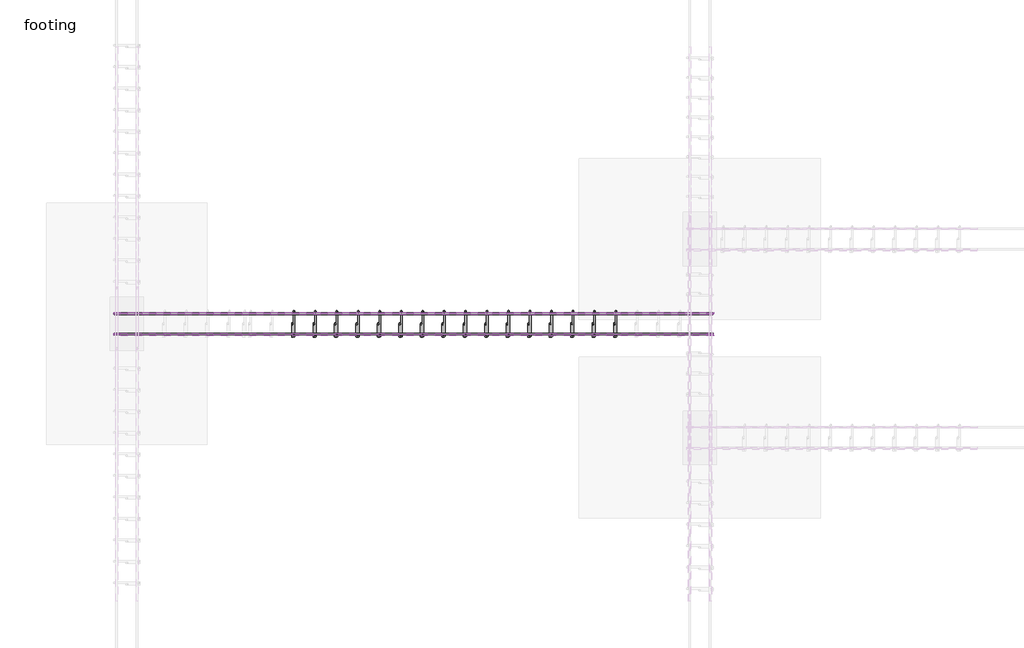
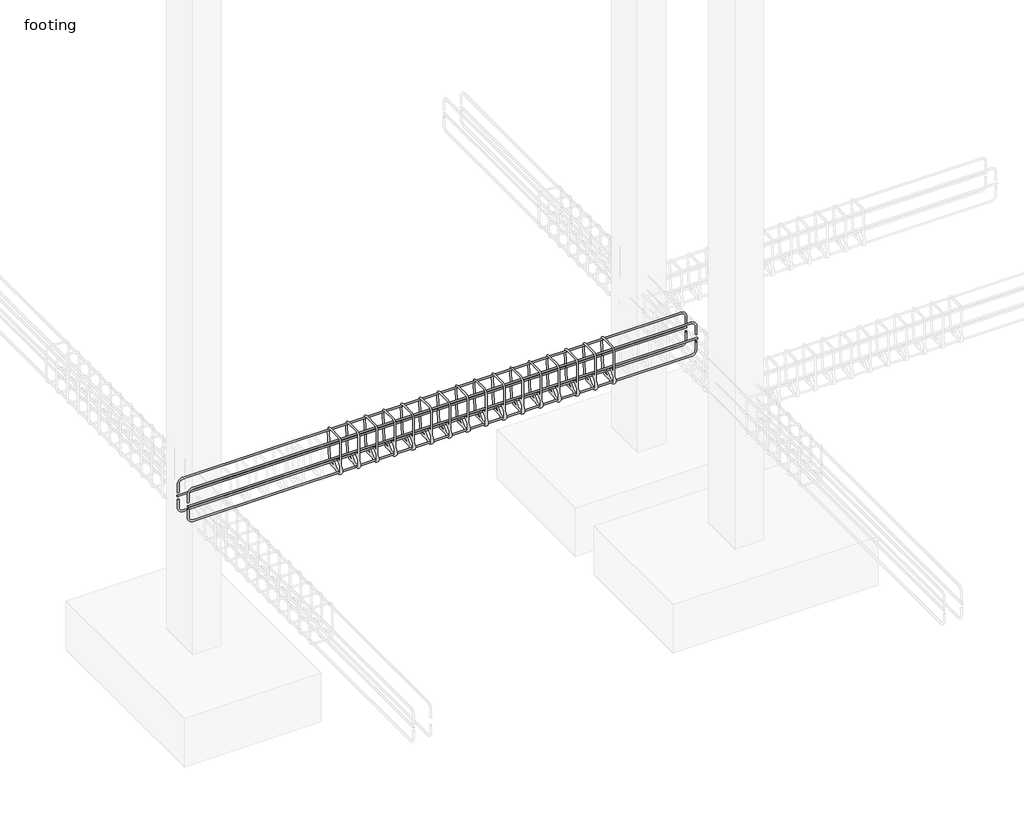
# One storey, part 8 of 21: 22 reinforcing bars.
"""IFC4 building model written with IfcOpenShell, lengths in millimetres."""

from ifc_helpers import new_model, si_unit, point, frame, origin, place, context, project, spatial, polyline, circle_curve, trimmed, segment, composite_curve, element, save
from ifc_brep_helpers import swept_disk

model = new_model("IFC4")

# Units and contexts
model_context = context("Model", 3, world=origin())
ifc_project = project(units=[si_unit("LENGTHUNIT", "METRE", prefix="MILLI")], contexts=[model_context])

# Site, building, storey
site = spatial("IfcSite", under=ifc_project)
building = spatial("IfcBuilding", under=site)
storey = spatial("IfcBuildingStorey", under=building, Name="footing", Elevation=-1524.0)

# Reinforcing bars
placement = place(None, origin())
element("IfcReinforcingBar", 1, at=placement, inside=storey, context=model_context, shape_type="SolidModel", body=[
    swept_disk(composite_curve([segment(polyline([(-10956.0883428, 7572.2887132, -310.8825168), (-10956.0883428, 7517.4237147, -365.7475153)]), True, "CONTINUOUS"), segment(trimmed(circle_curve(frame((-10956.0883428, 7494.9730744, -343.296875), z_axis=(-1.0, 0.0, 0.0), x_axis=(0.0, 22.450640300000487, -22.450640299999975)), 31.75), [point((-10956.0883428, 7517.4237147, -365.7475153))], [point((-10956.0883428, 7463.2230744, -343.296875))], True, "CARTESIAN"), True, "CONTINUOUS"), segment(polyline([(-10956.0883428, 7463.2230744, -343.296875), (-10956.0883428, 7463.2230744, -63.103125)]), True, "CONTINUOUS"), segment(trimmed(circle_curve(frame((-10956.0883428, 7494.9730744, -63.103125), z_axis=(-1.0, 0.0, 0.0), x_axis=(0.0, -31.75, 0.0)), 31.75), [point((-10956.0883428, 7463.2230744, -63.103125))], [point((-10956.0883428, 7494.9730744, -31.353125))], True, "CARTESIAN"), True, "CONTINUOUS"), segment(polyline([(-10956.0883428, 7494.9730744, -31.353125), (-10956.0883428, 7622.7668244, -31.353125)]), True, "CONTINUOUS"), segment(trimmed(circle_curve(frame((-10954.9159328, 7622.7668244, -63.0814712), z_axis=(-0.9993179916193466, 0.0, -0.03692629992126919), x_axis=(-1.1724099999992177, 0.0, 31.728346200000004)), 31.75), [point((-10956.0883428, 7622.7668244, -31.353125))], [point((-10954.9159328, 7654.5168244, -63.0814712))], True, "CARTESIAN"), True, "CONTINUOUS"), segment(polyline([(-10954.9159328, 7654.5168244, -63.0814712), (-10944.5607528, 7654.5168244, -343.3185288)]), True, "CONTINUOUS"), segment(trimmed(circle_curve(frame((-10944.5607528, 7622.7668244, -343.3185288), z_axis=(-0.9993179916193466, 0.0, -0.03692629992126919), x_axis=(0.0, 31.75, 0.0)), 31.75), [point((-10944.5607528, 7654.5168244, -343.3185288))], [point((-10943.3883428, 7622.7668244, -375.046875))], True, "CARTESIAN"), True, "CONTINUOUS"), segment(polyline([(-10943.3883428, 7622.7668244, -375.046875), (-10943.3883428, 7494.9730744, -375.046875)]), True, "CONTINUOUS"), segment(trimmed(circle_curve(frame((-10943.3883428, 7494.9730744, -343.296875), z_axis=(-1.0, 0.0, 0.0), x_axis=(0.0, 0.0, -31.75)), 31.75), [point((-10943.3883428, 7494.9730744, -375.046875))], [point((-10943.3883428, 7472.5224341, -320.8462347))], True, "CARTESIAN"), True, "CONTINUOUS"), segment(polyline([(-10943.3883428, 7472.5224341, -320.8462347), (-10943.3883428, 7527.3874326, -265.9812362)]), True, "CONTINUOUS")], self_intersect=False), 6.35),
])
element("IfcReinforcingBar", 2, at=placement, inside=storey, context=model_context, shape_type="SolidModel", body=[
    swept_disk(composite_curve([segment(polyline([(-10793.3883428, 7572.2887132, -310.8825168), (-10793.3883428, 7517.4237147, -365.7475153)]), True, "CONTINUOUS"), segment(trimmed(circle_curve(frame((-10793.3883428, 7494.9730744, -343.296875), z_axis=(-1.0, 0.0, 0.0), x_axis=(0.0, 22.450640300000487, -22.450640299999975)), 31.75), [point((-10793.3883428, 7517.4237147, -365.7475153))], [point((-10793.3883428, 7463.2230744, -343.296875))], True, "CARTESIAN"), True, "CONTINUOUS"), segment(polyline([(-10793.3883428, 7463.2230744, -343.296875), (-10793.3883428, 7463.2230744, -63.103125)]), True, "CONTINUOUS"), segment(trimmed(circle_curve(frame((-10793.3883428, 7494.9730744, -63.103125), z_axis=(-1.0, 0.0, 0.0), x_axis=(0.0, -31.75, 0.0)), 31.75), [point((-10793.3883428, 7463.2230744, -63.103125))], [point((-10793.3883428, 7494.9730744, -31.353125))], True, "CARTESIAN"), True, "CONTINUOUS"), segment(polyline([(-10793.3883428, 7494.9730744, -31.353125), (-10793.3883428, 7622.7668244, -31.353125)]), True, "CONTINUOUS"), segment(trimmed(circle_curve(frame((-10792.2159328, 7622.7668244, -63.0814712), z_axis=(-0.9993179916193466, 0.0, -0.03692629992126919), x_axis=(-1.1724100000010367, 0.0, 31.728346200000004)), 31.75), [point((-10793.3883428, 7622.7668244, -31.353125))], [point((-10792.2159328, 7654.5168244, -63.0814712))], True, "CARTESIAN"), True, "CONTINUOUS"), segment(polyline([(-10792.2159328, 7654.5168244, -63.0814712), (-10781.8607528, 7654.5168244, -343.3185288)]), True, "CONTINUOUS"), segment(trimmed(circle_curve(frame((-10781.8607528, 7622.7668244, -343.3185288), z_axis=(-0.9993179916193466, 0.0, -0.03692629992126919), x_axis=(0.0, 31.75, 0.0)), 31.75), [point((-10781.8607528, 7654.5168244, -343.3185288))], [point((-10780.6883428, 7622.7668244, -375.046875))], True, "CARTESIAN"), True, "CONTINUOUS"), segment(polyline([(-10780.6883428, 7622.7668244, -375.046875), (-10780.6883428, 7494.9730744, -375.046875)]), True, "CONTINUOUS"), segment(trimmed(circle_curve(frame((-10780.6883428, 7494.9730744, -343.296875), z_axis=(-1.0, 0.0, 0.0), x_axis=(0.0, 0.0, -31.75)), 31.75), [point((-10780.6883428, 7494.9730744, -375.046875))], [point((-10780.6883428, 7472.5224341, -320.8462347))], True, "CARTESIAN"), True, "CONTINUOUS"), segment(polyline([(-10780.6883428, 7472.5224341, -320.8462347), (-10780.6883428, 7527.3874326, -265.9812362)]), True, "CONTINUOUS")], self_intersect=False), 6.35),
])
element("IfcReinforcingBar", 3, at=placement, inside=storey, context=model_context, shape_type="SolidModel", body=[
    swept_disk(composite_curve([segment(polyline([(-10630.6883428, 7572.2887132, -310.8825168), (-10630.6883428, 7517.4237147, -365.7475153)]), True, "CONTINUOUS"), segment(trimmed(circle_curve(frame((-10630.6883428, 7494.9730744, -343.296875), z_axis=(-1.0, 0.0, 0.0), x_axis=(0.0, 22.450640300000487, -22.450640299999975)), 31.75), [point((-10630.6883428, 7517.4237147, -365.7475153))], [point((-10630.6883428, 7463.2230744, -343.296875))], True, "CARTESIAN"), True, "CONTINUOUS"), segment(polyline([(-10630.6883428, 7463.2230744, -343.296875), (-10630.6883428, 7463.2230744, -63.103125)]), True, "CONTINUOUS"), segment(trimmed(circle_curve(frame((-10630.6883428, 7494.9730744, -63.103125), z_axis=(-1.0, 0.0, 0.0), x_axis=(0.0, -31.75, 0.0)), 31.75), [point((-10630.6883428, 7463.2230744, -63.103125))], [point((-10630.6883428, 7494.9730744, -31.353125))], True, "CARTESIAN"), True, "CONTINUOUS"), segment(polyline([(-10630.6883428, 7494.9730744, -31.353125), (-10630.6883428, 7622.7668244, -31.353125)]), True, "CONTINUOUS"), segment(trimmed(circle_curve(frame((-10629.5159328, 7622.7668244, -63.0814712), z_axis=(-0.9993179916193466, 0.0, -0.03692629992126919), x_axis=(-1.1724099999992177, 0.0, 31.728346200000004)), 31.75), [point((-10630.6883428, 7622.7668244, -31.353125))], [point((-10629.5159328, 7654.5168244, -63.0814712))], True, "CARTESIAN"), True, "CONTINUOUS"), segment(polyline([(-10629.5159328, 7654.5168244, -63.0814712), (-10619.1607528, 7654.5168244, -343.3185288)]), True, "CONTINUOUS"), segment(trimmed(circle_curve(frame((-10619.1607528, 7622.7668244, -343.3185288), z_axis=(-0.9993179916193466, 0.0, -0.03692629992126919), x_axis=(0.0, 31.75, 0.0)), 31.75), [point((-10619.1607528, 7654.5168244, -343.3185288))], [point((-10617.9883428, 7622.7668244, -375.046875))], True, "CARTESIAN"), True, "CONTINUOUS"), segment(polyline([(-10617.9883428, 7622.7668244, -375.046875), (-10617.9883428, 7494.9730744, -375.046875)]), True, "CONTINUOUS"), segment(trimmed(circle_curve(frame((-10617.9883428, 7494.9730744, -343.296875), z_axis=(-1.0, 0.0, 0.0), x_axis=(0.0, 0.0, -31.75)), 31.75), [point((-10617.9883428, 7494.9730744, -375.046875))], [point((-10617.9883428, 7472.5224341, -320.8462347))], True, "CARTESIAN"), True, "CONTINUOUS"), segment(polyline([(-10617.9883428, 7472.5224341, -320.8462347), (-10617.9883428, 7527.3874326, -265.9812362)]), True, "CONTINUOUS")], self_intersect=False), 6.35),
])
element("IfcReinforcingBar", 4, at=placement, inside=storey, context=model_context, shape_type="SolidModel", body=[
    swept_disk(composite_curve([segment(polyline([(-10467.9883428, 7572.2887132, -310.8825168), (-10467.9883428, 7517.4237147, -365.7475153)]), True, "CONTINUOUS"), segment(trimmed(circle_curve(frame((-10467.9883428, 7494.9730744, -343.296875), z_axis=(-1.0, 0.0, 0.0), x_axis=(0.0, 22.450640300000487, -22.450640299999975)), 31.75), [point((-10467.9883428, 7517.4237147, -365.7475153))], [point((-10467.9883428, 7463.2230744, -343.296875))], True, "CARTESIAN"), True, "CONTINUOUS"), segment(polyline([(-10467.9883428, 7463.2230744, -343.296875), (-10467.9883428, 7463.2230744, -63.103125)]), True, "CONTINUOUS"), segment(trimmed(circle_curve(frame((-10467.9883428, 7494.9730744, -63.103125), z_axis=(-1.0, 0.0, 0.0), x_axis=(0.0, -31.75, 0.0)), 31.75), [point((-10467.9883428, 7463.2230744, -63.103125))], [point((-10467.9883428, 7494.9730744, -31.353125))], True, "CARTESIAN"), True, "CONTINUOUS"), segment(polyline([(-10467.9883428, 7494.9730744, -31.353125), (-10467.9883428, 7622.7668244, -31.353125)]), True, "CONTINUOUS"), segment(trimmed(circle_curve(frame((-10466.8159328, 7622.7668244, -63.0814712), z_axis=(-0.9993179916193466, 0.0, -0.03692629992126919), x_axis=(-1.1724099999992177, 0.0, 31.728346200000004)), 31.75), [point((-10467.9883428, 7622.7668244, -31.353125))], [point((-10466.8159328, 7654.5168244, -63.0814712))], True, "CARTESIAN"), True, "CONTINUOUS"), segment(polyline([(-10466.8159328, 7654.5168244, -63.0814712), (-10456.4607528, 7654.5168244, -343.3185288)]), True, "CONTINUOUS"), segment(trimmed(circle_curve(frame((-10456.4607528, 7622.7668244, -343.3185288), z_axis=(-0.9993179916193466, 0.0, -0.03692629992126919), x_axis=(0.0, 31.75, 0.0)), 31.75), [point((-10456.4607528, 7654.5168244, -343.3185288))], [point((-10455.2883428, 7622.7668244, -375.046875))], True, "CARTESIAN"), True, "CONTINUOUS"), segment(polyline([(-10455.2883428, 7622.7668244, -375.046875), (-10455.2883428, 7494.9730744, -375.046875)]), True, "CONTINUOUS"), segment(trimmed(circle_curve(frame((-10455.2883428, 7494.9730744, -343.296875), z_axis=(-1.0, 0.0, 0.0), x_axis=(0.0, 0.0, -31.75)), 31.75), [point((-10455.2883428, 7494.9730744, -375.046875))], [point((-10455.2883428, 7472.5224341, -320.8462347))], True, "CARTESIAN"), True, "CONTINUOUS"), segment(polyline([(-10455.2883428, 7472.5224341, -320.8462347), (-10455.2883428, 7527.3874326, -265.9812362)]), True, "CONTINUOUS")], self_intersect=False), 6.35),
])
element("IfcReinforcingBar", 5, at=placement, inside=storey, context=model_context, shape_type="SolidModel", body=[
    swept_disk(composite_curve([segment(polyline([(-10305.2883428, 7572.2887132, -310.8825168), (-10305.2883428, 7517.4237147, -365.7475153)]), True, "CONTINUOUS"), segment(trimmed(circle_curve(frame((-10305.2883428, 7494.9730744, -343.296875), z_axis=(-1.0, 0.0, 0.0), x_axis=(0.0, 22.450640300000487, -22.450640299999975)), 31.75), [point((-10305.2883428, 7517.4237147, -365.7475153))], [point((-10305.2883428, 7463.2230744, -343.296875))], True, "CARTESIAN"), True, "CONTINUOUS"), segment(polyline([(-10305.2883428, 7463.2230744, -343.296875), (-10305.2883428, 7463.2230744, -63.103125)]), True, "CONTINUOUS"), segment(trimmed(circle_curve(frame((-10305.2883428, 7494.9730744, -63.103125), z_axis=(-1.0, 0.0, 0.0), x_axis=(0.0, -31.75, 0.0)), 31.75), [point((-10305.2883428, 7463.2230744, -63.103125))], [point((-10305.2883428, 7494.9730744, -31.353125))], True, "CARTESIAN"), True, "CONTINUOUS"), segment(polyline([(-10305.2883428, 7494.9730744, -31.353125), (-10305.2883428, 7622.7668244, -31.353125)]), True, "CONTINUOUS"), segment(trimmed(circle_curve(frame((-10304.1159328, 7622.7668244, -63.0814712), z_axis=(-0.9993179916193466, 0.0, -0.03692629992126919), x_axis=(-1.1724100000010367, 0.0, 31.728346200000004)), 31.75), [point((-10305.2883428, 7622.7668244, -31.353125))], [point((-10304.1159328, 7654.5168244, -63.0814712))], True, "CARTESIAN"), True, "CONTINUOUS"), segment(polyline([(-10304.1159328, 7654.5168244, -63.0814712), (-10293.7607528, 7654.5168244, -343.3185288)]), True, "CONTINUOUS"), segment(trimmed(circle_curve(frame((-10293.7607528, 7622.7668244, -343.3185288), z_axis=(-0.9993179916193466, 0.0, -0.03692629992126919), x_axis=(0.0, 31.75, 0.0)), 31.75), [point((-10293.7607528, 7654.5168244, -343.3185288))], [point((-10292.5883428, 7622.7668244, -375.046875))], True, "CARTESIAN"), True, "CONTINUOUS"), segment(polyline([(-10292.5883428, 7622.7668244, -375.046875), (-10292.5883428, 7494.9730744, -375.046875)]), True, "CONTINUOUS"), segment(trimmed(circle_curve(frame((-10292.5883428, 7494.9730744, -343.296875), z_axis=(-1.0, 0.0, 0.0), x_axis=(0.0, 0.0, -31.75)), 31.75), [point((-10292.5883428, 7494.9730744, -375.046875))], [point((-10292.5883428, 7472.5224341, -320.8462347))], True, "CARTESIAN"), True, "CONTINUOUS"), segment(polyline([(-10292.5883428, 7472.5224341, -320.8462347), (-10292.5883428, 7527.3874326, -265.9812362)]), True, "CONTINUOUS")], self_intersect=False), 6.35),
])
element("IfcReinforcingBar", 6, at=placement, inside=storey, context=model_context, shape_type="SolidModel", body=[
    swept_disk(composite_curve([segment(polyline([(-10142.5883428, 7572.2887132, -310.8825168), (-10142.5883428, 7517.4237147, -365.7475153)]), True, "CONTINUOUS"), segment(trimmed(circle_curve(frame((-10142.5883428, 7494.9730744, -343.296875), z_axis=(-1.0, 0.0, 0.0), x_axis=(0.0, 22.450640300000487, -22.450640299999975)), 31.75), [point((-10142.5883428, 7517.4237147, -365.7475153))], [point((-10142.5883428, 7463.2230744, -343.296875))], True, "CARTESIAN"), True, "CONTINUOUS"), segment(polyline([(-10142.5883428, 7463.2230744, -343.296875), (-10142.5883428, 7463.2230744, -63.103125)]), True, "CONTINUOUS"), segment(trimmed(circle_curve(frame((-10142.5883428, 7494.9730744, -63.103125), z_axis=(-1.0, 0.0, 0.0), x_axis=(0.0, -31.75, 0.0)), 31.75), [point((-10142.5883428, 7463.2230744, -63.103125))], [point((-10142.5883428, 7494.9730744, -31.353125))], True, "CARTESIAN"), True, "CONTINUOUS"), segment(polyline([(-10142.5883428, 7494.9730744, -31.353125), (-10142.5883428, 7622.7668244, -31.353125)]), True, "CONTINUOUS"), segment(trimmed(circle_curve(frame((-10141.4159328, 7622.7668244, -63.0814712), z_axis=(-0.9993179916193466, 0.0, -0.03692629992126919), x_axis=(-1.1724099999992177, 0.0, 31.728346200000004)), 31.75), [point((-10142.5883428, 7622.7668244, -31.353125))], [point((-10141.4159328, 7654.5168244, -63.0814712))], True, "CARTESIAN"), True, "CONTINUOUS"), segment(polyline([(-10141.4159328, 7654.5168244, -63.0814712), (-10131.0607528, 7654.5168244, -343.3185288)]), True, "CONTINUOUS"), segment(trimmed(circle_curve(frame((-10131.0607528, 7622.7668244, -343.3185288), z_axis=(-0.9993179916193466, 0.0, -0.03692629992126919), x_axis=(0.0, 31.75, 0.0)), 31.75), [point((-10131.0607528, 7654.5168244, -343.3185288))], [point((-10129.8883428, 7622.7668244, -375.046875))], True, "CARTESIAN"), True, "CONTINUOUS"), segment(polyline([(-10129.8883428, 7622.7668244, -375.046875), (-10129.8883428, 7494.9730744, -375.046875)]), True, "CONTINUOUS"), segment(trimmed(circle_curve(frame((-10129.8883428, 7494.9730744, -343.296875), z_axis=(-1.0, 0.0, 0.0), x_axis=(0.0, 0.0, -31.75)), 31.75), [point((-10129.8883428, 7494.9730744, -375.046875))], [point((-10129.8883428, 7472.5224341, -320.8462347))], True, "CARTESIAN"), True, "CONTINUOUS"), segment(polyline([(-10129.8883428, 7472.5224341, -320.8462347), (-10129.8883428, 7527.3874326, -265.9812362)]), True, "CONTINUOUS")], self_intersect=False), 6.35),
])
element("IfcReinforcingBar", 7, at=placement, inside=storey, context=model_context, shape_type="SolidModel", body=[
    swept_disk(composite_curve([segment(polyline([(-9979.8883428, 7572.2887132, -310.8825168), (-9979.8883428, 7517.4237147, -365.7475153)]), True, "CONTINUOUS"), segment(trimmed(circle_curve(frame((-9979.8883428, 7494.9730744, -343.296875), z_axis=(-1.0, 0.0, 0.0), x_axis=(0.0, 22.450640300000487, -22.450640299999975)), 31.75), [point((-9979.8883428, 7517.4237147, -365.7475153))], [point((-9979.8883428, 7463.2230744, -343.296875))], True, "CARTESIAN"), True, "CONTINUOUS"), segment(polyline([(-9979.8883428, 7463.2230744, -343.296875), (-9979.8883428, 7463.2230744, -63.103125)]), True, "CONTINUOUS"), segment(trimmed(circle_curve(frame((-9979.8883428, 7494.9730744, -63.103125), z_axis=(-1.0, 0.0, 0.0), x_axis=(0.0, -31.75, 0.0)), 31.75), [point((-9979.8883428, 7463.2230744, -63.103125))], [point((-9979.8883428, 7494.9730744, -31.353125))], True, "CARTESIAN"), True, "CONTINUOUS"), segment(polyline([(-9979.8883428, 7494.9730744, -31.353125), (-9979.8883428, 7622.7668244, -31.353125)]), True, "CONTINUOUS"), segment(trimmed(circle_curve(frame((-9978.7159328, 7622.7668244, -63.0814712), z_axis=(-0.9993179916193466, 0.0, -0.03692629992126919), x_axis=(-1.1724100000010367, 0.0, 31.728346200000004)), 31.75), [point((-9979.8883428, 7622.7668244, -31.353125))], [point((-9978.7159328, 7654.5168244, -63.0814712))], True, "CARTESIAN"), True, "CONTINUOUS"), segment(polyline([(-9978.7159328, 7654.5168244, -63.0814712), (-9968.3607528, 7654.5168244, -343.3185288)]), True, "CONTINUOUS"), segment(trimmed(circle_curve(frame((-9968.3607528, 7622.7668244, -343.3185288), z_axis=(-0.9993179916193466, 0.0, -0.03692629992126919), x_axis=(0.0, 31.75, 0.0)), 31.75), [point((-9968.3607528, 7654.5168244, -343.3185288))], [point((-9967.1883428, 7622.7668244, -375.046875))], True, "CARTESIAN"), True, "CONTINUOUS"), segment(polyline([(-9967.1883428, 7622.7668244, -375.046875), (-9967.1883428, 7494.9730744, -375.046875)]), True, "CONTINUOUS"), segment(trimmed(circle_curve(frame((-9967.1883428, 7494.9730744, -343.296875), z_axis=(-1.0, 0.0, 0.0), x_axis=(0.0, 0.0, -31.75)), 31.75), [point((-9967.1883428, 7494.9730744, -375.046875))], [point((-9967.1883428, 7472.5224341, -320.8462347))], True, "CARTESIAN"), True, "CONTINUOUS"), segment(polyline([(-9967.1883428, 7472.5224341, -320.8462347), (-9967.1883428, 7527.3874326, -265.9812362)]), True, "CONTINUOUS")], self_intersect=False), 6.35),
])
element("IfcReinforcingBar", 8, at=placement, inside=storey, context=model_context, shape_type="SolidModel", body=[
    swept_disk(composite_curve([segment(polyline([(-9817.1883428, 7572.2887132, -310.8825168), (-9817.1883428, 7517.4237147, -365.7475153)]), True, "CONTINUOUS"), segment(trimmed(circle_curve(frame((-9817.1883428, 7494.9730744, -343.296875), z_axis=(-1.0, 0.0, 0.0), x_axis=(0.0, 22.450640300000487, -22.450640299999975)), 31.75), [point((-9817.1883428, 7517.4237147, -365.7475153))], [point((-9817.1883428, 7463.2230744, -343.296875))], True, "CARTESIAN"), True, "CONTINUOUS"), segment(polyline([(-9817.1883428, 7463.2230744, -343.296875), (-9817.1883428, 7463.2230744, -63.103125)]), True, "CONTINUOUS"), segment(trimmed(circle_curve(frame((-9817.1883428, 7494.9730744, -63.103125), z_axis=(-1.0, 0.0, 0.0), x_axis=(0.0, -31.75, 0.0)), 31.75), [point((-9817.1883428, 7463.2230744, -63.103125))], [point((-9817.1883428, 7494.9730744, -31.353125))], True, "CARTESIAN"), True, "CONTINUOUS"), segment(polyline([(-9817.1883428, 7494.9730744, -31.353125), (-9817.1883428, 7622.7668244, -31.353125)]), True, "CONTINUOUS"), segment(trimmed(circle_curve(frame((-9816.0159328, 7622.7668244, -63.0814712), z_axis=(-0.9993179916193466, 0.0, -0.03692629992126919), x_axis=(-1.1724099999992177, 0.0, 31.728346200000004)), 31.75), [point((-9817.1883428, 7622.7668244, -31.353125))], [point((-9816.0159328, 7654.5168244, -63.0814712))], True, "CARTESIAN"), True, "CONTINUOUS"), segment(polyline([(-9816.0159328, 7654.5168244, -63.0814712), (-9805.6607528, 7654.5168244, -343.3185288)]), True, "CONTINUOUS"), segment(trimmed(circle_curve(frame((-9805.6607528, 7622.7668244, -343.3185288), z_axis=(-0.9993179916193466, 0.0, -0.03692629992126919), x_axis=(0.0, 31.75, 0.0)), 31.75), [point((-9805.6607528, 7654.5168244, -343.3185288))], [point((-9804.4883428, 7622.7668244, -375.046875))], True, "CARTESIAN"), True, "CONTINUOUS"), segment(polyline([(-9804.4883428, 7622.7668244, -375.046875), (-9804.4883428, 7494.9730744, -375.046875)]), True, "CONTINUOUS"), segment(trimmed(circle_curve(frame((-9804.4883428, 7494.9730744, -343.296875), z_axis=(-1.0, 0.0, 0.0), x_axis=(0.0, 0.0, -31.75)), 31.75), [point((-9804.4883428, 7494.9730744, -375.046875))], [point((-9804.4883428, 7472.5224341, -320.8462347))], True, "CARTESIAN"), True, "CONTINUOUS"), segment(polyline([(-9804.4883428, 7472.5224341, -320.8462347), (-9804.4883428, 7527.3874326, -265.9812362)]), True, "CONTINUOUS")], self_intersect=False), 6.35),
])
element("IfcReinforcingBar", 9, at=placement, inside=storey, context=model_context, shape_type="SolidModel", body=[
    swept_disk(composite_curve([segment(polyline([(-9654.4883428, 7572.2887132, -310.8825168), (-9654.4883428, 7517.4237147, -365.7475153)]), True, "CONTINUOUS"), segment(trimmed(circle_curve(frame((-9654.4883428, 7494.9730744, -343.296875), z_axis=(-1.0, 0.0, 0.0), x_axis=(0.0, 22.450640300000487, -22.450640299999975)), 31.75), [point((-9654.4883428, 7517.4237147, -365.7475153))], [point((-9654.4883428, 7463.2230744, -343.296875))], True, "CARTESIAN"), True, "CONTINUOUS"), segment(polyline([(-9654.4883428, 7463.2230744, -343.296875), (-9654.4883428, 7463.2230744, -63.103125)]), True, "CONTINUOUS"), segment(trimmed(circle_curve(frame((-9654.4883428, 7494.9730744, -63.103125), z_axis=(-1.0, 0.0, 0.0), x_axis=(0.0, -31.75, 0.0)), 31.75), [point((-9654.4883428, 7463.2230744, -63.103125))], [point((-9654.4883428, 7494.9730744, -31.353125))], True, "CARTESIAN"), True, "CONTINUOUS"), segment(polyline([(-9654.4883428, 7494.9730744, -31.353125), (-9654.4883428, 7622.7668244, -31.353125)]), True, "CONTINUOUS"), segment(trimmed(circle_curve(frame((-9653.3159328, 7622.7668244, -63.0814712), z_axis=(-0.9993179916193466, 0.0, -0.03692629992126919), x_axis=(-1.1724099999992177, 0.0, 31.728346200000004)), 31.75), [point((-9654.4883428, 7622.7668244, -31.353125))], [point((-9653.3159328, 7654.5168244, -63.0814712))], True, "CARTESIAN"), True, "CONTINUOUS"), segment(polyline([(-9653.3159328, 7654.5168244, -63.0814712), (-9642.9607528, 7654.5168244, -343.3185288)]), True, "CONTINUOUS"), segment(trimmed(circle_curve(frame((-9642.9607528, 7622.7668244, -343.3185288), z_axis=(-0.9993179916193466, 0.0, -0.03692629992126919), x_axis=(0.0, 31.75, 0.0)), 31.75), [point((-9642.9607528, 7654.5168244, -343.3185288))], [point((-9641.7883428, 7622.7668244, -375.046875))], True, "CARTESIAN"), True, "CONTINUOUS"), segment(polyline([(-9641.7883428, 7622.7668244, -375.046875), (-9641.7883428, 7494.9730744, -375.046875)]), True, "CONTINUOUS"), segment(trimmed(circle_curve(frame((-9641.7883428, 7494.9730744, -343.296875), z_axis=(-1.0, 0.0, 0.0), x_axis=(0.0, 0.0, -31.75)), 31.75), [point((-9641.7883428, 7494.9730744, -375.046875))], [point((-9641.7883428, 7472.5224341, -320.8462347))], True, "CARTESIAN"), True, "CONTINUOUS"), segment(polyline([(-9641.7883428, 7472.5224341, -320.8462347), (-9641.7883428, 7527.3874326, -265.9812362)]), True, "CONTINUOUS")], self_intersect=False), 6.35),
])
element("IfcReinforcingBar", 10, at=placement, inside=storey, context=model_context, shape_type="SolidModel", body=[
    swept_disk(composite_curve([segment(polyline([(-9491.7883428, 7572.2887132, -310.8825168), (-9491.7883428, 7517.4237147, -365.7475153)]), True, "CONTINUOUS"), segment(trimmed(circle_curve(frame((-9491.7883428, 7494.9730744, -343.296875), z_axis=(-1.0, 0.0, 0.0), x_axis=(0.0, 22.450640300000487, -22.450640299999975)), 31.75), [point((-9491.7883428, 7517.4237147, -365.7475153))], [point((-9491.7883428, 7463.2230744, -343.296875))], True, "CARTESIAN"), True, "CONTINUOUS"), segment(polyline([(-9491.7883428, 7463.2230744, -343.296875), (-9491.7883428, 7463.2230744, -63.103125)]), True, "CONTINUOUS"), segment(trimmed(circle_curve(frame((-9491.7883428, 7494.9730744, -63.103125), z_axis=(-1.0, 0.0, 0.0), x_axis=(0.0, -31.75, 0.0)), 31.75), [point((-9491.7883428, 7463.2230744, -63.103125))], [point((-9491.7883428, 7494.9730744, -31.353125))], True, "CARTESIAN"), True, "CONTINUOUS"), segment(polyline([(-9491.7883428, 7494.9730744, -31.353125), (-9491.7883428, 7622.7668244, -31.353125)]), True, "CONTINUOUS"), segment(trimmed(circle_curve(frame((-9490.6159328, 7622.7668244, -63.0814712), z_axis=(-0.9993179916193466, 0.0, -0.03692629992126919), x_axis=(-1.1724100000010367, 0.0, 31.728346200000004)), 31.75), [point((-9491.7883428, 7622.7668244, -31.353125))], [point((-9490.6159328, 7654.5168244, -63.0814712))], True, "CARTESIAN"), True, "CONTINUOUS"), segment(polyline([(-9490.6159328, 7654.5168244, -63.0814712), (-9480.2607528, 7654.5168244, -343.3185288)]), True, "CONTINUOUS"), segment(trimmed(circle_curve(frame((-9480.2607528, 7622.7668244, -343.3185288), z_axis=(-0.9993179916193466, 0.0, -0.03692629992126919), x_axis=(0.0, 31.75, 0.0)), 31.75), [point((-9480.2607528, 7654.5168244, -343.3185288))], [point((-9479.0883428, 7622.7668244, -375.046875))], True, "CARTESIAN"), True, "CONTINUOUS"), segment(polyline([(-9479.0883428, 7622.7668244, -375.046875), (-9479.0883428, 7494.9730744, -375.046875)]), True, "CONTINUOUS"), segment(trimmed(circle_curve(frame((-9479.0883428, 7494.9730744, -343.296875), z_axis=(-1.0, 0.0, 0.0), x_axis=(0.0, 0.0, -31.75)), 31.75), [point((-9479.0883428, 7494.9730744, -375.046875))], [point((-9479.0883428, 7472.5224341, -320.8462347))], True, "CARTESIAN"), True, "CONTINUOUS"), segment(polyline([(-9479.0883428, 7472.5224341, -320.8462347), (-9479.0883428, 7527.3874326, -265.9812362)]), True, "CONTINUOUS")], self_intersect=False), 6.35),
])
element("IfcReinforcingBar", 11, at=placement, inside=storey, context=model_context, shape_type="SolidModel", body=[
    swept_disk(composite_curve([segment(polyline([(-9329.0883428, 7572.2887132, -310.8825168), (-9329.0883428, 7517.4237147, -365.7475153)]), True, "CONTINUOUS"), segment(trimmed(circle_curve(frame((-9329.0883428, 7494.9730744, -343.296875), z_axis=(-1.0, 0.0, 0.0), x_axis=(0.0, 22.450640300000487, -22.450640299999975)), 31.75), [point((-9329.0883428, 7517.4237147, -365.7475153))], [point((-9329.0883428, 7463.2230744, -343.296875))], True, "CARTESIAN"), True, "CONTINUOUS"), segment(polyline([(-9329.0883428, 7463.2230744, -343.296875), (-9329.0883428, 7463.2230744, -63.103125)]), True, "CONTINUOUS"), segment(trimmed(circle_curve(frame((-9329.0883428, 7494.9730744, -63.103125), z_axis=(-1.0, 0.0, 0.0), x_axis=(0.0, -31.75, 0.0)), 31.75), [point((-9329.0883428, 7463.2230744, -63.103125))], [point((-9329.0883428, 7494.9730744, -31.353125))], True, "CARTESIAN"), True, "CONTINUOUS"), segment(polyline([(-9329.0883428, 7494.9730744, -31.353125), (-9329.0883428, 7622.7668244, -31.353125)]), True, "CONTINUOUS"), segment(trimmed(circle_curve(frame((-9327.9159328, 7622.7668244, -63.0814712), z_axis=(-0.9993179916193466, 0.0, -0.03692629992126919), x_axis=(-1.1724099999992177, 0.0, 31.728346200000004)), 31.75), [point((-9329.0883428, 7622.7668244, -31.353125))], [point((-9327.9159328, 7654.5168244, -63.0814712))], True, "CARTESIAN"), True, "CONTINUOUS"), segment(polyline([(-9327.9159328, 7654.5168244, -63.0814712), (-9317.5607528, 7654.5168244, -343.3185288)]), True, "CONTINUOUS"), segment(trimmed(circle_curve(frame((-9317.5607528, 7622.7668244, -343.3185288), z_axis=(-0.9993179916193466, 0.0, -0.03692629992126919), x_axis=(0.0, 31.75, 0.0)), 31.75), [point((-9317.5607528, 7654.5168244, -343.3185288))], [point((-9316.3883428, 7622.7668244, -375.046875))], True, "CARTESIAN"), True, "CONTINUOUS"), segment(polyline([(-9316.3883428, 7622.7668244, -375.046875), (-9316.3883428, 7494.9730744, -375.046875)]), True, "CONTINUOUS"), segment(trimmed(circle_curve(frame((-9316.3883428, 7494.9730744, -343.296875), z_axis=(-1.0, 0.0, 0.0), x_axis=(0.0, 0.0, -31.75)), 31.75), [point((-9316.3883428, 7494.9730744, -375.046875))], [point((-9316.3883428, 7472.5224341, -320.8462347))], True, "CARTESIAN"), True, "CONTINUOUS"), segment(polyline([(-9316.3883428, 7472.5224341, -320.8462347), (-9316.3883428, 7527.3874326, -265.9812362)]), True, "CONTINUOUS")], self_intersect=False), 6.35),
])
element("IfcReinforcingBar", 12, at=placement, inside=storey, context=model_context, shape_type="SolidModel", body=[
    swept_disk(composite_curve([segment(polyline([(-9166.3883428, 7572.2887132, -310.8825168), (-9166.3883428, 7517.4237147, -365.7475153)]), True, "CONTINUOUS"), segment(trimmed(circle_curve(frame((-9166.3883428, 7494.9730744, -343.296875), z_axis=(-1.0, 0.0, 0.0), x_axis=(0.0, 22.450640300000487, -22.450640299999975)), 31.75), [point((-9166.3883428, 7517.4237147, -365.7475153))], [point((-9166.3883428, 7463.2230744, -343.296875))], True, "CARTESIAN"), True, "CONTINUOUS"), segment(polyline([(-9166.3883428, 7463.2230744, -343.296875), (-9166.3883428, 7463.2230744, -63.103125)]), True, "CONTINUOUS"), segment(trimmed(circle_curve(frame((-9166.3883428, 7494.9730744, -63.103125), z_axis=(-1.0, 0.0, 0.0), x_axis=(0.0, -31.75, 0.0)), 31.75), [point((-9166.3883428, 7463.2230744, -63.103125))], [point((-9166.3883428, 7494.9730744, -31.353125))], True, "CARTESIAN"), True, "CONTINUOUS"), segment(polyline([(-9166.3883428, 7494.9730744, -31.353125), (-9166.3883428, 7622.7668244, -31.353125)]), True, "CONTINUOUS"), segment(trimmed(circle_curve(frame((-9165.2159328, 7622.7668244, -63.0814712), z_axis=(-0.9993179916193466, 0.0, -0.03692629992126919), x_axis=(-1.1724100000010367, 0.0, 31.728346200000004)), 31.75), [point((-9166.3883428, 7622.7668244, -31.353125))], [point((-9165.2159328, 7654.5168244, -63.0814712))], True, "CARTESIAN"), True, "CONTINUOUS"), segment(polyline([(-9165.2159328, 7654.5168244, -63.0814712), (-9154.8607528, 7654.5168244, -343.3185288)]), True, "CONTINUOUS"), segment(trimmed(circle_curve(frame((-9154.8607528, 7622.7668244, -343.3185288), z_axis=(-0.9993179916193466, 0.0, -0.03692629992126919), x_axis=(0.0, 31.75, 0.0)), 31.75), [point((-9154.8607528, 7654.5168244, -343.3185288))], [point((-9153.6883428, 7622.7668244, -375.046875))], True, "CARTESIAN"), True, "CONTINUOUS"), segment(polyline([(-9153.6883428, 7622.7668244, -375.046875), (-9153.6883428, 7494.9730744, -375.046875)]), True, "CONTINUOUS"), segment(trimmed(circle_curve(frame((-9153.6883428, 7494.9730744, -343.296875), z_axis=(-1.0, 0.0, 0.0), x_axis=(0.0, 0.0, -31.75)), 31.75), [point((-9153.6883428, 7494.9730744, -375.046875))], [point((-9153.6883428, 7472.5224341, -320.8462347))], True, "CARTESIAN"), True, "CONTINUOUS"), segment(polyline([(-9153.6883428, 7472.5224341, -320.8462347), (-9153.6883428, 7527.3874326, -265.9812362)]), True, "CONTINUOUS")], self_intersect=False), 6.35),
])
element("IfcReinforcingBar", 13, at=placement, inside=storey, context=model_context, shape_type="SolidModel", body=[
    swept_disk(composite_curve([segment(polyline([(-9003.6883428, 7572.2887132, -310.8825168), (-9003.6883428, 7517.4237147, -365.7475153)]), True, "CONTINUOUS"), segment(trimmed(circle_curve(frame((-9003.6883428, 7494.9730744, -343.296875), z_axis=(-1.0, 0.0, 0.0), x_axis=(0.0, 22.450640300000487, -22.450640299999975)), 31.75), [point((-9003.6883428, 7517.4237147, -365.7475153))], [point((-9003.6883428, 7463.2230744, -343.296875))], True, "CARTESIAN"), True, "CONTINUOUS"), segment(polyline([(-9003.6883428, 7463.2230744, -343.296875), (-9003.6883428, 7463.2230744, -63.103125)]), True, "CONTINUOUS"), segment(trimmed(circle_curve(frame((-9003.6883428, 7494.9730744, -63.103125), z_axis=(-1.0, 0.0, 0.0), x_axis=(0.0, -31.75, 0.0)), 31.75), [point((-9003.6883428, 7463.2230744, -63.103125))], [point((-9003.6883428, 7494.9730744, -31.353125))], True, "CARTESIAN"), True, "CONTINUOUS"), segment(polyline([(-9003.6883428, 7494.9730744, -31.353125), (-9003.6883428, 7622.7668244, -31.353125)]), True, "CONTINUOUS"), segment(trimmed(circle_curve(frame((-9002.5159328, 7622.7668244, -63.0814712), z_axis=(-0.9993179916193466, 0.0, -0.03692629992126919), x_axis=(-1.1724099999992177, 0.0, 31.728346200000004)), 31.75), [point((-9003.6883428, 7622.7668244, -31.353125))], [point((-9002.5159328, 7654.5168244, -63.0814712))], True, "CARTESIAN"), True, "CONTINUOUS"), segment(polyline([(-9002.5159328, 7654.5168244, -63.0814712), (-8992.1607528, 7654.5168244, -343.3185288)]), True, "CONTINUOUS"), segment(trimmed(circle_curve(frame((-8992.1607528, 7622.7668244, -343.3185288), z_axis=(-0.9993179916193466, 0.0, -0.03692629992126919), x_axis=(0.0, 31.75, 0.0)), 31.75), [point((-8992.1607528, 7654.5168244, -343.3185288))], [point((-8990.9883428, 7622.7668244, -375.046875))], True, "CARTESIAN"), True, "CONTINUOUS"), segment(polyline([(-8990.9883428, 7622.7668244, -375.046875), (-8990.9883428, 7494.9730744, -375.046875)]), True, "CONTINUOUS"), segment(trimmed(circle_curve(frame((-8990.9883428, 7494.9730744, -343.296875), z_axis=(-1.0, 0.0, 0.0), x_axis=(0.0, 0.0, -31.75)), 31.75), [point((-8990.9883428, 7494.9730744, -375.046875))], [point((-8990.9883428, 7472.5224341, -320.8462347))], True, "CARTESIAN"), True, "CONTINUOUS"), segment(polyline([(-8990.9883428, 7472.5224341, -320.8462347), (-8990.9883428, 7527.3874326, -265.9812362)]), True, "CONTINUOUS")], self_intersect=False), 6.35),
])
element("IfcReinforcingBar", 14, at=placement, inside=storey, context=model_context, shape_type="SolidModel", body=[
    swept_disk(composite_curve([segment(polyline([(-8840.9883428, 7572.2887132, -310.8825168), (-8840.9883428, 7517.4237147, -365.7475153)]), True, "CONTINUOUS"), segment(trimmed(circle_curve(frame((-8840.9883428, 7494.9730744, -343.296875), z_axis=(-1.0, 0.0, 0.0), x_axis=(0.0, 22.450640300000487, -22.450640299999975)), 31.75), [point((-8840.9883428, 7517.4237147, -365.7475153))], [point((-8840.9883428, 7463.2230744, -343.296875))], True, "CARTESIAN"), True, "CONTINUOUS"), segment(polyline([(-8840.9883428, 7463.2230744, -343.296875), (-8840.9883428, 7463.2230744, -63.103125)]), True, "CONTINUOUS"), segment(trimmed(circle_curve(frame((-8840.9883428, 7494.9730744, -63.103125), z_axis=(-1.0, 0.0, 0.0), x_axis=(0.0, -31.75, 0.0)), 31.75), [point((-8840.9883428, 7463.2230744, -63.103125))], [point((-8840.9883428, 7494.9730744, -31.353125))], True, "CARTESIAN"), True, "CONTINUOUS"), segment(polyline([(-8840.9883428, 7494.9730744, -31.353125), (-8840.9883428, 7622.7668244, -31.353125)]), True, "CONTINUOUS"), segment(trimmed(circle_curve(frame((-8839.8159328, 7622.7668244, -63.0814712), z_axis=(-0.9993179916193466, 0.0, -0.03692629992126919), x_axis=(-1.1724099999992177, 0.0, 31.728346200000004)), 31.75), [point((-8840.9883428, 7622.7668244, -31.353125))], [point((-8839.8159328, 7654.5168244, -63.0814712))], True, "CARTESIAN"), True, "CONTINUOUS"), segment(polyline([(-8839.8159328, 7654.5168244, -63.0814712), (-8829.4607528, 7654.5168244, -343.3185288)]), True, "CONTINUOUS"), segment(trimmed(circle_curve(frame((-8829.4607528, 7622.7668244, -343.3185288), z_axis=(-0.9993179916193466, 0.0, -0.03692629992126919), x_axis=(0.0, 31.75, 0.0)), 31.75), [point((-8829.4607528, 7654.5168244, -343.3185288))], [point((-8828.2883428, 7622.7668244, -375.046875))], True, "CARTESIAN"), True, "CONTINUOUS"), segment(polyline([(-8828.2883428, 7622.7668244, -375.046875), (-8828.2883428, 7494.9730744, -375.046875)]), True, "CONTINUOUS"), segment(trimmed(circle_curve(frame((-8828.2883428, 7494.9730744, -343.296875), z_axis=(-1.0, 0.0, 0.0), x_axis=(0.0, 0.0, -31.75)), 31.75), [point((-8828.2883428, 7494.9730744, -375.046875))], [point((-8828.2883428, 7472.5224341, -320.8462347))], True, "CARTESIAN"), True, "CONTINUOUS"), segment(polyline([(-8828.2883428, 7472.5224341, -320.8462347), (-8828.2883428, 7527.3874326, -265.9812362)]), True, "CONTINUOUS")], self_intersect=False), 6.35),
])
element("IfcReinforcingBar", 15, at=placement, inside=storey, context=model_context, shape_type="SolidModel", body=[
    swept_disk(composite_curve([segment(polyline([(-8678.2883428, 7572.2887132, -310.8825168), (-8678.2883428, 7517.4237147, -365.7475153)]), True, "CONTINUOUS"), segment(trimmed(circle_curve(frame((-8678.2883428, 7494.9730744, -343.296875), z_axis=(-1.0, 0.0, 0.0), x_axis=(0.0, 22.450640300000487, -22.450640299999975)), 31.75), [point((-8678.2883428, 7517.4237147, -365.7475153))], [point((-8678.2883428, 7463.2230744, -343.296875))], True, "CARTESIAN"), True, "CONTINUOUS"), segment(polyline([(-8678.2883428, 7463.2230744, -343.296875), (-8678.2883428, 7463.2230744, -63.103125)]), True, "CONTINUOUS"), segment(trimmed(circle_curve(frame((-8678.2883428, 7494.9730744, -63.103125), z_axis=(-1.0, 0.0, 0.0), x_axis=(0.0, -31.75, 0.0)), 31.75), [point((-8678.2883428, 7463.2230744, -63.103125))], [point((-8678.2883428, 7494.9730744, -31.353125))], True, "CARTESIAN"), True, "CONTINUOUS"), segment(polyline([(-8678.2883428, 7494.9730744, -31.353125), (-8678.2883428, 7622.7668244, -31.353125)]), True, "CONTINUOUS"), segment(trimmed(circle_curve(frame((-8677.1159328, 7622.7668244, -63.0814712), z_axis=(-0.9993179916193466, 0.0, -0.03692629992126919), x_axis=(-1.1724100000010367, 0.0, 31.728346200000004)), 31.75), [point((-8678.2883428, 7622.7668244, -31.353125))], [point((-8677.1159328, 7654.5168244, -63.0814712))], True, "CARTESIAN"), True, "CONTINUOUS"), segment(polyline([(-8677.1159328, 7654.5168244, -63.0814712), (-8666.7607528, 7654.5168244, -343.3185288)]), True, "CONTINUOUS"), segment(trimmed(circle_curve(frame((-8666.7607528, 7622.7668244, -343.3185288), z_axis=(-0.9993179916193466, 0.0, -0.03692629992126919), x_axis=(0.0, 31.75, 0.0)), 31.75), [point((-8666.7607528, 7654.5168244, -343.3185288))], [point((-8665.5883428, 7622.7668244, -375.046875))], True, "CARTESIAN"), True, "CONTINUOUS"), segment(polyline([(-8665.5883428, 7622.7668244, -375.046875), (-8665.5883428, 7494.9730744, -375.046875)]), True, "CONTINUOUS"), segment(trimmed(circle_curve(frame((-8665.5883428, 7494.9730744, -343.296875), z_axis=(-1.0, 0.0, 0.0), x_axis=(0.0, 0.0, -31.75)), 31.75), [point((-8665.5883428, 7494.9730744, -375.046875))], [point((-8665.5883428, 7472.5224341, -320.8462347))], True, "CARTESIAN"), True, "CONTINUOUS"), segment(polyline([(-8665.5883428, 7472.5224341, -320.8462347), (-8665.5883428, 7527.3874326, -265.9812362)]), True, "CONTINUOUS")], self_intersect=False), 6.35),
])
element("IfcReinforcingBar", 16, at=placement, inside=storey, context=model_context, shape_type="SolidModel", body=[
    swept_disk(composite_curve([segment(polyline([(-8515.5883428, 7572.2887132, -310.8825168), (-8515.5883428, 7517.4237147, -365.7475153)]), True, "CONTINUOUS"), segment(trimmed(circle_curve(frame((-8515.5883428, 7494.9730744, -343.296875), z_axis=(-1.0, 0.0, 0.0), x_axis=(0.0, 22.450640300000487, -22.450640299999975)), 31.75), [point((-8515.5883428, 7517.4237147, -365.7475153))], [point((-8515.5883428, 7463.2230744, -343.296875))], True, "CARTESIAN"), True, "CONTINUOUS"), segment(polyline([(-8515.5883428, 7463.2230744, -343.296875), (-8515.5883428, 7463.2230744, -63.103125)]), True, "CONTINUOUS"), segment(trimmed(circle_curve(frame((-8515.5883428, 7494.9730744, -63.103125), z_axis=(-1.0, 0.0, 0.0), x_axis=(0.0, -31.75, 0.0)), 31.75), [point((-8515.5883428, 7463.2230744, -63.103125))], [point((-8515.5883428, 7494.9730744, -31.353125))], True, "CARTESIAN"), True, "CONTINUOUS"), segment(polyline([(-8515.5883428, 7494.9730744, -31.353125), (-8515.5883428, 7622.7668244, -31.353125)]), True, "CONTINUOUS"), segment(trimmed(circle_curve(frame((-8514.4159328, 7622.7668244, -63.0814712), z_axis=(-0.9993179916193466, 0.0, -0.03692629992126919), x_axis=(-1.1724099999992177, 0.0, 31.728346200000004)), 31.75), [point((-8515.5883428, 7622.7668244, -31.353125))], [point((-8514.4159328, 7654.5168244, -63.0814712))], True, "CARTESIAN"), True, "CONTINUOUS"), segment(polyline([(-8514.4159328, 7654.5168244, -63.0814712), (-8504.0607528, 7654.5168244, -343.3185288)]), True, "CONTINUOUS"), segment(trimmed(circle_curve(frame((-8504.0607528, 7622.7668244, -343.3185288), z_axis=(-0.9993179916193466, 0.0, -0.03692629992126919), x_axis=(0.0, 31.75, 0.0)), 31.75), [point((-8504.0607528, 7654.5168244, -343.3185288))], [point((-8502.8883428, 7622.7668244, -375.046875))], True, "CARTESIAN"), True, "CONTINUOUS"), segment(polyline([(-8502.8883428, 7622.7668244, -375.046875), (-8502.8883428, 7494.9730744, -375.046875)]), True, "CONTINUOUS"), segment(trimmed(circle_curve(frame((-8502.8883428, 7494.9730744, -343.296875), z_axis=(-1.0, 0.0, 0.0), x_axis=(0.0, 0.0, -31.75)), 31.75), [point((-8502.8883428, 7494.9730744, -375.046875))], [point((-8502.8883428, 7472.5224341, -320.8462347))], True, "CARTESIAN"), True, "CONTINUOUS"), segment(polyline([(-8502.8883428, 7472.5224341, -320.8462347), (-8502.8883428, 7527.3874326, -265.9812362)]), True, "CONTINUOUS")], self_intersect=False), 6.35),
])
element("IfcReinforcingBar", 17, at=placement, inside=storey, context=model_context, shape_type="SolidModel", body=[
    swept_disk(composite_curve([segment(polyline([(-7770.5521673, 7636.2372086, -236.1172592), (-7770.5521673, 7636.2372086, -312.3172592)]), True, "CONTINUOUS"), segment(trimmed(circle_curve(frame((-7815.0021673, 7636.2372086, -312.3172592), z_axis=(0.0, 1.0, -2.1166279873208456e-12), x_axis=(44.44999999999982, 0.0, 0.0)), 44.45), [point((-7770.5521673, 7636.2372086, -312.3172592))], [point((-7815.0021673, 7636.2372086, -356.7672592))], True, "CARTESIAN"), True, "CONTINUOUS"), segment(polyline([(-7815.0021673, 7636.2372086, -356.7672592), (-12260.7959173, 7636.2372086, -356.7672592)]), True, "CONTINUOUS"), segment(trimmed(circle_curve(frame((-12260.7959173, 7636.2372086, -312.3172592), z_axis=(0.0, 1.0, -2.1166279873208456e-12), x_axis=(0.0, 0.0, -44.44999999999999)), 44.45), [point((-12260.7959173, 7636.2372086, -356.7672592))], [point((-12305.2459173, 7636.2372086, -312.3172592))], True, "CARTESIAN"), True, "CONTINUOUS"), segment(polyline([(-12305.2459173, 7636.2372086, -312.3172592), (-12305.2459173, 7636.2372086, -236.1172592)]), True, "CONTINUOUS")], self_intersect=False), 6.35),
])
element("IfcReinforcingBar", 18, at=placement, inside=storey, context=model_context, shape_type="SolidModel", body=[
    swept_disk(composite_curve([segment(polyline([(-7770.5521673, 7481.5026902, -170.2827408), (-7770.5521673, 7481.5026902, -94.0827408)]), True, "CONTINUOUS"), segment(trimmed(circle_curve(frame((-7815.0021673, 7481.5026902, -94.0827408), z_axis=(0.0, -1.0, 0.0), x_axis=(44.44999999999982, 0.0, 0.0)), 44.45), [point((-7770.5521673, 7481.5026902, -94.0827408))], [point((-7815.0021673, 7481.5026902, -49.6327408))], True, "CARTESIAN"), True, "CONTINUOUS"), segment(polyline([(-7815.0021673, 7481.5026902, -49.6327408), (-12260.7959173, 7481.5026902, -49.6327408)]), True, "CONTINUOUS"), segment(trimmed(circle_curve(frame((-12260.7959173, 7481.5026902, -94.0827408), z_axis=(0.0, -1.0, 0.0), x_axis=(0.0, 0.0, 44.449999999999996)), 44.45), [point((-12260.7959173, 7481.5026902, -49.6327408))], [point((-12305.2459173, 7481.5026902, -94.0827408))], True, "CARTESIAN"), True, "CONTINUOUS"), segment(polyline([(-12305.2459173, 7481.5026902, -94.0827408), (-12305.2459173, 7481.5026902, -170.2827408)]), True, "CONTINUOUS")], self_intersect=False), 6.35),
])
element("IfcReinforcingBar", 19, at=placement, inside=storey, context=model_context, shape_type="SolidModel", body=[
    swept_disk(composite_curve([segment(polyline([(-7770.5521673, 7481.5026902, -236.1172592), (-7770.5521673, 7481.5026902, -312.3172592)]), True, "CONTINUOUS"), segment(trimmed(circle_curve(frame((-7815.0021673, 7481.5026902, -312.3172592), z_axis=(0.0, 1.0, 2.1166279873208456e-12), x_axis=(44.44999999999982, 0.0, 0.0)), 44.45), [point((-7770.5521673, 7481.5026902, -312.3172592))], [point((-7815.0021673, 7481.5026902, -356.7672592))], True, "CARTESIAN"), True, "CONTINUOUS"), segment(polyline([(-7815.0021673, 7481.5026902, -356.7672592), (-12260.7959173, 7481.5026902, -356.7672592)]), True, "CONTINUOUS"), segment(trimmed(circle_curve(frame((-12260.7959173, 7481.5026902, -312.3172592), z_axis=(0.0, 1.0, 2.1166279873208456e-12), x_axis=(0.0, 0.0, -44.44999999999999)), 44.45), [point((-12260.7959173, 7481.5026902, -356.7672592))], [point((-12305.2459173, 7481.5026902, -312.3172592))], True, "CARTESIAN"), True, "CONTINUOUS"), segment(polyline([(-12305.2459173, 7481.5026902, -312.3172592), (-12305.2459173, 7481.5026902, -236.1172592)]), True, "CONTINUOUS")], self_intersect=False), 6.35),
])
element("IfcReinforcingBar", 20, at=placement, inside=storey, context=model_context, shape_type="SolidModel", body=[
    swept_disk(composite_curve([segment(polyline([(-7770.5521673, 7636.2372086, -170.2827408), (-7770.5521673, 7636.2372086, -94.0827408)]), True, "CONTINUOUS"), segment(trimmed(circle_curve(frame((-7815.0021673, 7636.2372086, -94.0827408), z_axis=(0.0, -1.0, 0.0), x_axis=(44.44999999999982, 0.0, 0.0)), 44.45), [point((-7770.5521673, 7636.2372086, -94.0827408))], [point((-7815.0021673, 7636.2372086, -49.6327408))], True, "CARTESIAN"), True, "CONTINUOUS"), segment(polyline([(-7815.0021673, 7636.2372086, -49.6327408), (-12260.7959173, 7636.2372086, -49.6327408)]), True, "CONTINUOUS"), segment(trimmed(circle_curve(frame((-12260.7959173, 7636.2372086, -94.0827408), z_axis=(0.0, -1.0, 0.0), x_axis=(0.0, 0.0, 44.449999999999996)), 44.45), [point((-12260.7959173, 7636.2372086, -49.6327408))], [point((-12305.2459173, 7636.2372086, -94.0827408))], True, "CARTESIAN"), True, "CONTINUOUS"), segment(polyline([(-12305.2459173, 7636.2372086, -94.0827408), (-12305.2459173, 7636.2372086, -170.2827408)]), True, "CONTINUOUS")], self_intersect=False), 6.35),
])
element("IfcReinforcingBar", 21, at=placement, inside=storey, context=model_context, shape_type="SolidModel", body=[
    swept_disk(composite_curve([segment(polyline([(-7764.2021673, 7641.8168244, -203.2), (-12311.5959173, 7641.8168244, -203.2)]), True, "CONTINUOUS")], self_intersect=False), 6.35),
])
element("IfcReinforcingBar", 22, at=placement, inside=storey, context=model_context, shape_type="SolidModel", body=[
    swept_disk(composite_curve([segment(polyline([(-7764.2021673, 7475.9230744, -203.2), (-12311.5959173, 7475.9230744, -203.2)]), True, "CONTINUOUS")], self_intersect=False), 6.35),
])

save(model, "model.ifc")

# Revit data of these elements
# Elements 1, 2, 3, 4, 5, 6, 7, 8, 9, 10, 11, 12, 13, 14, 15, 16, 17, 18, 19, 20, 21, 22 (IfcReinforcingBar)
#   Phase Created = New Construction
